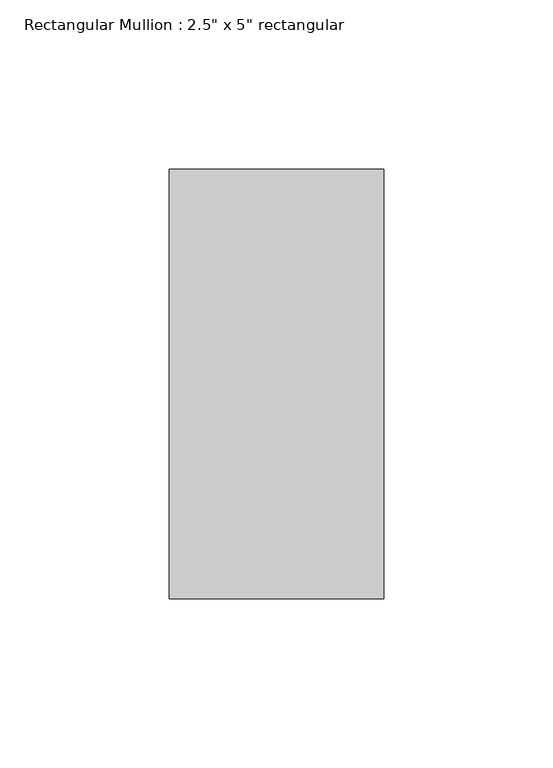
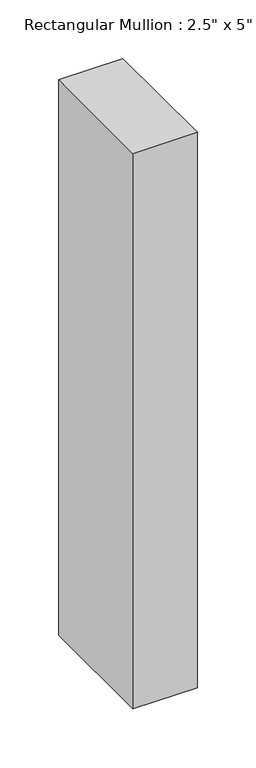
"""IFC4 building model written with IfcOpenShell, lengths in millimetres: member geometry."""

from ifc_helpers import new_model, si_unit, frame, origin, place, context, project, spatial, polyline, outline, extrude, source, transform, mapped, element, save


def member_912d8bb3(model_context):
    return source(origin(), model_context, "Body", "SweptSolid", [
        extrude(outline(polyline([(0.0, 63.5), (0.0, -63.5), (-63.5, -63.5), (-63.5, 63.5), (0.0, 63.5)])), frame((0.0, 0.0, -579.9666667), z_axis=(0.0, 0.0, 1.0), x_axis=(1.0, 0.0, 0.0)), (0.0, 0.0, 1.0), 579.9666667),
    ])


if __name__ == "__main__":
    model = new_model("IFC4")
    model_context = context("Model", 3, world=origin())
    ifc_project = project(units=[si_unit("LENGTHUNIT", "METRE", prefix="MILLI")], contexts=[model_context])
    site = spatial("IfcSite", under=ifc_project)
    building = spatial("IfcBuilding", under=site)
    placement = place(None, origin())
    member_shape = member_912d8bb3(model_context)
    element("IfcMember", 1, ObjectType="Rectangular Mullion : 2.5\" x 5\" rectangular", at=placement, inside=building, context=model_context, shape_type="MappedRepresentation", body=[
        mapped(member_shape, transform((0.0, 0.0, 0.0), x_axis=(1.0, 0.0, 0.0), y_axis=(0.0, 1.0, 0.0), z_axis=(0.0, 0.0, 1.0))),
    ])
    save(model, "model.ifc")

# Revit data of these elements
# Type "Rectangular Mullion : 2.5\" x 5\" rectangular"
#   built-in parameter 1007304 = 0.416667 (stored number, unit not read)
#   built-in parameter 1007301 = 0.104167 (stored number, unit not read)
#   built-in parameter 1007300 = 0.104167 (stored number, unit not read)
# Element 1 (IfcMember, "Rectangular Mullion : 2.5\" x 5\" rectangular")
#   Materials on its faces: "Aluminum"
# Materials
#   "Aluminum": class "Metal", colour RGB 247 247 247, transparency 0, Description = "Aluminum 6061", Cost = 0
